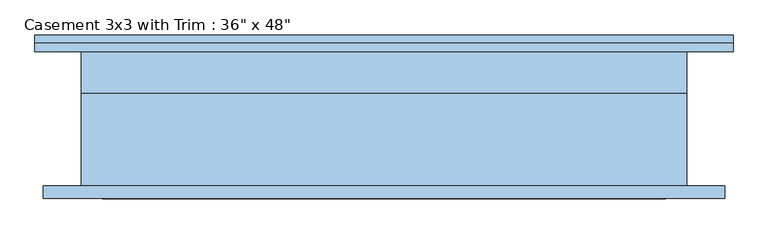
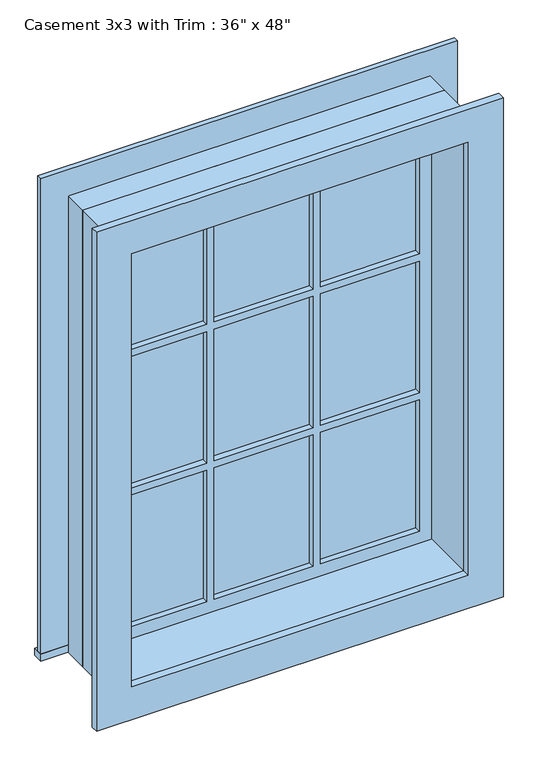
"""IFC4 building model written with IfcOpenShell, lengths in millimetres: window geometry."""

from ifc_helpers import new_model, si_unit, frame, origin, place, context, project, spatial, polyline, outline, extrude, source, transform, mapped, element, save


def window_29c06734(model_context):
    return source(origin(), model_context, "Body", "SweptSolid", [
        extrude(outline(polyline([(-527.05, 127.0), (527.05, 127.0), (527.05, 101.6), (-527.05, 101.6), (-527.05, 127.0)])), frame((0.0, 0.0, 914.4), z_axis=(0.0, 0.0, 1.0), x_axis=(1.0, 0.0, 0.0)), (0.0, 0.0, 1.0), 19.05),
        extrude(outline(polyline([(2114.55, -438.15), (2114.55, 438.15), (933.45, 438.15), (933.45, 527.05), (2203.45, 527.05), (2203.45, -527.05), (933.45, -527.05), (933.45, -438.15), (2114.55, -438.15)])), frame((0.0, 101.6, 0.0), z_axis=(0.0, 1.0, 0.0), x_axis=(0.0, 0.0, 1.0)), (0.0, 0.0, 1.0), 12.7),
        extrude(outline(polyline([(143.9333333, 66.675), (393.7, 66.675), (393.7, 53.975), (143.9333333, 53.975), (143.9333333, 66.675)])), frame((0.0, 0.0, 1718.7333333), z_axis=(0.0, 0.0, 1.0), x_axis=(1.0, 0.0, 0.0)), (0.0, 0.0, 1.0), 351.3666667),
        extrude(outline(polyline([(-124.8833333, 66.675), (124.8833333, 66.675), (124.8833333, 53.975), (-124.8833333, 53.975), (-124.8833333, 66.675)])), frame((0.0, 0.0, 1718.7333333), z_axis=(0.0, 0.0, 1.0), x_axis=(1.0, 0.0, 0.0)), (0.0, 0.0, 1.0), 351.3666667),
        extrude(outline(polyline([(-393.7, 66.675), (-143.9333333, 66.675), (-143.9333333, 53.975), (-393.7, 53.975), (-393.7, 66.675)])), frame((0.0, 0.0, 1718.7333333), z_axis=(0.0, 0.0, 1.0), x_axis=(1.0, 0.0, 0.0)), (0.0, 0.0, 1.0), 351.3666667),
        extrude(outline(polyline([(-393.7, 66.675), (-143.9333333, 66.675), (-143.9333333, 53.975), (-393.7, 53.975), (-393.7, 66.675)])), frame((0.0, 0.0, 1348.3166667), z_axis=(0.0, 0.0, 1.0), x_axis=(1.0, 0.0, 0.0)), (0.0, 0.0, 1.0), 351.3666667),
        extrude(outline(polyline([(-124.8833333, 66.675), (124.8833333, 66.675), (124.8833333, 53.975), (-124.8833333, 53.975), (-124.8833333, 66.675)])), frame((0.0, 0.0, 1348.3166667), z_axis=(0.0, 0.0, 1.0), x_axis=(1.0, 0.0, 0.0)), (0.0, 0.0, 1.0), 351.3666667),
        extrude(outline(polyline([(143.9333333, 66.675), (393.7, 66.675), (393.7, 53.975), (143.9333333, 53.975), (143.9333333, 66.675)])), frame((0.0, 0.0, 1348.3166667), z_axis=(0.0, 0.0, 1.0), x_axis=(1.0, 0.0, 0.0)), (0.0, 0.0, 1.0), 351.3666667),
        extrude(outline(polyline([(143.9333333, 66.675), (393.7, 66.675), (393.7, 53.975), (143.9333333, 53.975), (143.9333333, 66.675)])), frame((0.0, 0.0, 977.9), z_axis=(0.0, 0.0, 1.0), x_axis=(1.0, 0.0, 0.0)), (0.0, 0.0, 1.0), 351.3666667),
        extrude(outline(polyline([(-124.8833333, 66.675), (124.8833333, 66.675), (124.8833333, 53.975), (-124.8833333, 53.975), (-124.8833333, 66.675)])), frame((0.0, 0.0, 977.9), z_axis=(0.0, 0.0, 1.0), x_axis=(1.0, 0.0, 0.0)), (0.0, 0.0, 1.0), 351.3666667),
        extrude(outline(polyline([(-393.7, 66.675), (-143.9333333, 66.675), (-143.9333333, 53.975), (-393.7, 53.975), (-393.7, 66.675)])), frame((0.0, 0.0, 977.9), z_axis=(0.0, 0.0, 1.0), x_axis=(1.0, 0.0, 0.0)), (0.0, 0.0, 1.0), 351.3666667),
        extrude(outline(polyline([(2190.75, 514.35), (2190.75, -514.35), (857.25, -514.35), (857.25, 514.35), (2190.75, 514.35)]), holes=[polyline([(2101.85, 425.45), (946.15, 425.45), (946.15, -425.45), (2101.85, -425.45), (2101.85, 425.45)])]), frame((0.0, -120.65, 0.0), z_axis=(0.0, 1.0, 0.0), x_axis=(0.0, 0.0, 1.0)), (0.0, 0.0, 1.0), 19.05),
        extrude(outline(polyline([(2114.55, -438.15), (933.45, -438.15), (933.45, 438.15), (2114.55, 438.15), (2114.55, -438.15)]), holes=[polyline([(2070.1, -143.9333333), (1718.7333333, -143.9333333), (1718.7333333, -393.7), (2070.1, -393.7), (2070.1, -143.9333333)]), polyline([(1699.6833333, -143.9333333), (1348.3166667, -143.9333333), (1348.3166667, -393.7), (1699.6833333, -393.7), (1699.6833333, -143.9333333)]), polyline([(1329.2666667, -143.9333333), (977.9, -143.9333333), (977.9, -393.7), (1329.2666667, -393.7), (1329.2666667, -143.9333333)]), polyline([(2070.1, 124.8833333), (1718.7333333, 124.8833333), (1718.7333333, -124.8833333), (2070.1, -124.8833333), (2070.1, 124.8833333)]), polyline([(1699.6833333, 124.8833333), (1348.3166667, 124.8833333), (1348.3166667, -124.8833333), (1699.6833333, -124.8833333), (1699.6833333, 124.8833333)]), polyline([(1329.2666667, 124.8833333), (977.9, 124.8833333), (977.9, -124.8833333), (1329.2666667, -124.8833333), (1329.2666667, 124.8833333)]), polyline([(2070.1, 393.7), (1718.7333333, 393.7), (1718.7333333, 143.9333333), (2070.1, 143.9333333), (2070.1, 393.7)]), polyline([(1699.6833333, 393.7), (1348.3166667, 393.7), (1348.3166667, 143.9333333), (1699.6833333, 143.9333333), (1699.6833333, 393.7)]), polyline([(1329.2666667, 393.7), (977.9, 393.7), (977.9, 143.9333333), (1329.2666667, 143.9333333), (1329.2666667, 393.7)])]), frame((0.0, 38.1, 0.0), z_axis=(0.0, 1.0, 0.0), x_axis=(0.0, 0.0, 1.0)), (0.0, 0.0, 1.0), 44.45),
        extrude(outline(polyline([(2133.6, -457.2), (914.4, -457.2), (914.4, 457.2), (2133.6, 457.2), (2133.6, -457.2)]), holes=[polyline([(2101.85, -425.45), (2101.85, 425.45), (946.15, 425.45), (946.15, -425.45), (2101.85, -425.45)])]), frame((0.0, -101.6, 0.0), z_axis=(0.0, 1.0, 0.0), x_axis=(0.0, 0.0, 1.0)), (0.0, 0.0, 1.0), 139.7),
        extrude(outline(polyline([(2133.6, 457.2), (2133.6, -457.2), (914.4, -457.2), (914.4, 457.2), (2133.6, 457.2)]), holes=[polyline([(2114.55, 438.15), (933.45, 438.15), (933.45, -438.15), (2114.55, -438.15), (2114.55, 438.15)])]), frame((0.0, 38.1, 0.0), z_axis=(0.0, 1.0, 0.0), x_axis=(0.0, 0.0, 1.0)), (0.0, 0.0, 1.0), 63.5),
    ])


if __name__ == "__main__":
    model = new_model("IFC4")
    model_context = context("Model", 3, world=origin())
    ifc_project = project(units=[si_unit("LENGTHUNIT", "METRE", prefix="MILLI")], contexts=[model_context])
    site = spatial("IfcSite", under=ifc_project)
    building = spatial("IfcBuilding", under=site)
    placement = place(None, origin())
    window_shape = window_29c06734(model_context)
    element("IfcWindow", 1, ObjectType="Casement 3x3 with Trim : 36\" x 48\"", at=placement, inside=building, context=model_context, shape_type="MappedRepresentation", body=[
        mapped(window_shape, transform((0.0, 0.0, 0.0), x_axis=(1.0, 0.0, 0.0), y_axis=(0.0, 1.0, 0.0), z_axis=(0.0, 0.0, 1.0))),
    ])
    save(model, "model.ifc")

# Revit data of these elements
# Type "Casement 3x3 with Trim : 36\" x 48\""
#   Type Mark = "21"
#   Construction Type Id = "GSP4R"
#   Assembly Code = "B2020100"
#   Analytic Construction = "1/8 in Pilkington single glazing"
#   Visual Light Transmittance = 0.9
#   Solar Heat Gain Coefficient = 0.78
#   Heat Transfer Coefficient (U) = 0.6496 BTU/(h·ft²·°F)
#   Height = 4' - 0"
#   Default Sill Height = 3' - 0"
#   Trim Projection - Ext. = 0' - 0 1/2"
#   Trim Projection - Int. = 0' - 0 3/4"
#   Trim Width - Exterior = 0' - 3 1/2"
#   Trim Width - Interior = 0' - 3 1/2"
#   Width = 3' - 0"
#   Window Inset = 0' - 0 3/4"
#   Define Thermal Properties by = 1
#   Glass Pane Material = Glass
#   Sash Material = Sash
#   Trim Exterior Material = Trim
#   Trim Interior Material = Trim
#   Wall Closure = (empty or 0)
# Element 1 (IfcWindow, "Casement 3x3 with Trim : 36\" x 48\"")
#   Materials on its faces: "Sash", "Glass", "Trim"
# Materials
#   "Glass": class "Glass", colour RGB 0 128 192, transparency 0.75, Description = "Soda Lime Glass", Cost = 0
#   "Sash": class "Wood", colour RGB 224 178 126, transparency 0
#   "Trim": class "Wood", colour RGB 224 178 126, transparency 0
